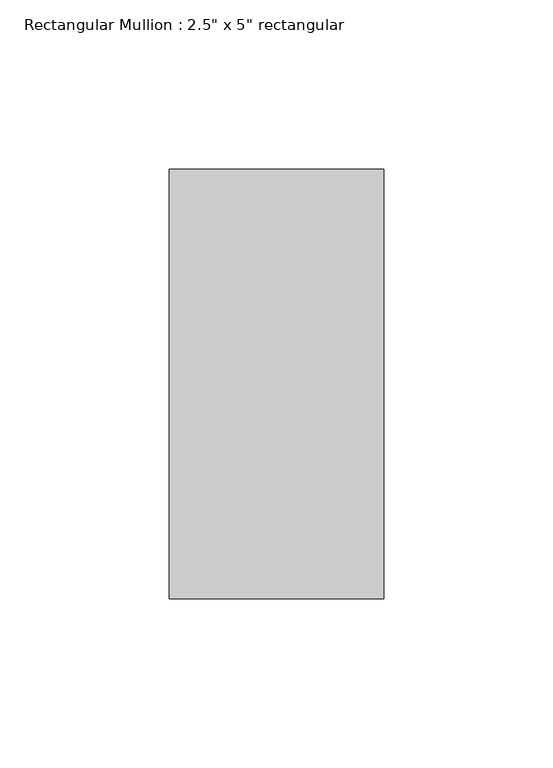
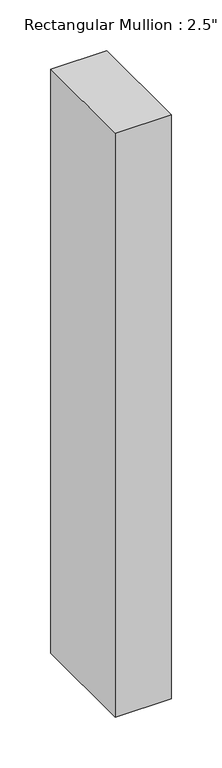
"""IFC4 building model written with IfcOpenShell, lengths in millimetres: member geometry."""

from ifc_helpers import new_model, si_unit, frame, origin, place, context, project, spatial, polyline, outline, extrude, source, transform, mapped, element, save


def member_dfbe4da1(model_context):
    return source(origin(), model_context, "Body", "SweptSolid", [
        extrude(outline(polyline([(0.0, 63.5), (0.0, -63.5), (-63.5, -63.5), (-63.5, 63.5), (0.0, 63.5)])), frame((0.0, 0.0, -702.226051), z_axis=(0.0, 0.0, 1.0), x_axis=(1.0, 0.0, 0.0)), (0.0, 0.0, 1.0), 702.226051),
    ])


if __name__ == "__main__":
    model = new_model("IFC4")
    model_context = context("Model", 3, world=origin())
    ifc_project = project(units=[si_unit("LENGTHUNIT", "METRE", prefix="MILLI")], contexts=[model_context])
    site = spatial("IfcSite", under=ifc_project)
    building = spatial("IfcBuilding", under=site)
    placement = place(None, origin())
    member_shape = member_dfbe4da1(model_context)
    element("IfcMember", 1, ObjectType="Rectangular Mullion : 2.5\" x 5\" rectangular", at=placement, inside=building, context=model_context, shape_type="MappedRepresentation", body=[
        mapped(member_shape, transform((0.0, 0.0, 0.0), x_axis=(1.0, 0.0, 0.0), y_axis=(0.0, 1.0, 0.0), z_axis=(0.0, 0.0, 1.0))),
    ])
    save(model, "model.ifc")

# Revit data of these elements
# Type "Rectangular Mullion : 2.5\" x 5\" rectangular"
#   built-in parameter 1007304 = 0.416667 (stored number, unit not read)
#   built-in parameter 1007301 = 0.104167 (stored number, unit not read)
#   built-in parameter 1007300 = 0.104167 (stored number, unit not read)
# Element 1 (IfcMember, "Rectangular Mullion : 2.5\" x 5\" rectangular")
#   Materials on its faces: "Aluminum"
# Materials
#   "Aluminum": class "Metal", colour RGB 247 247 247, transparency 0, Description = "Aluminum 6061", Cost = 0
